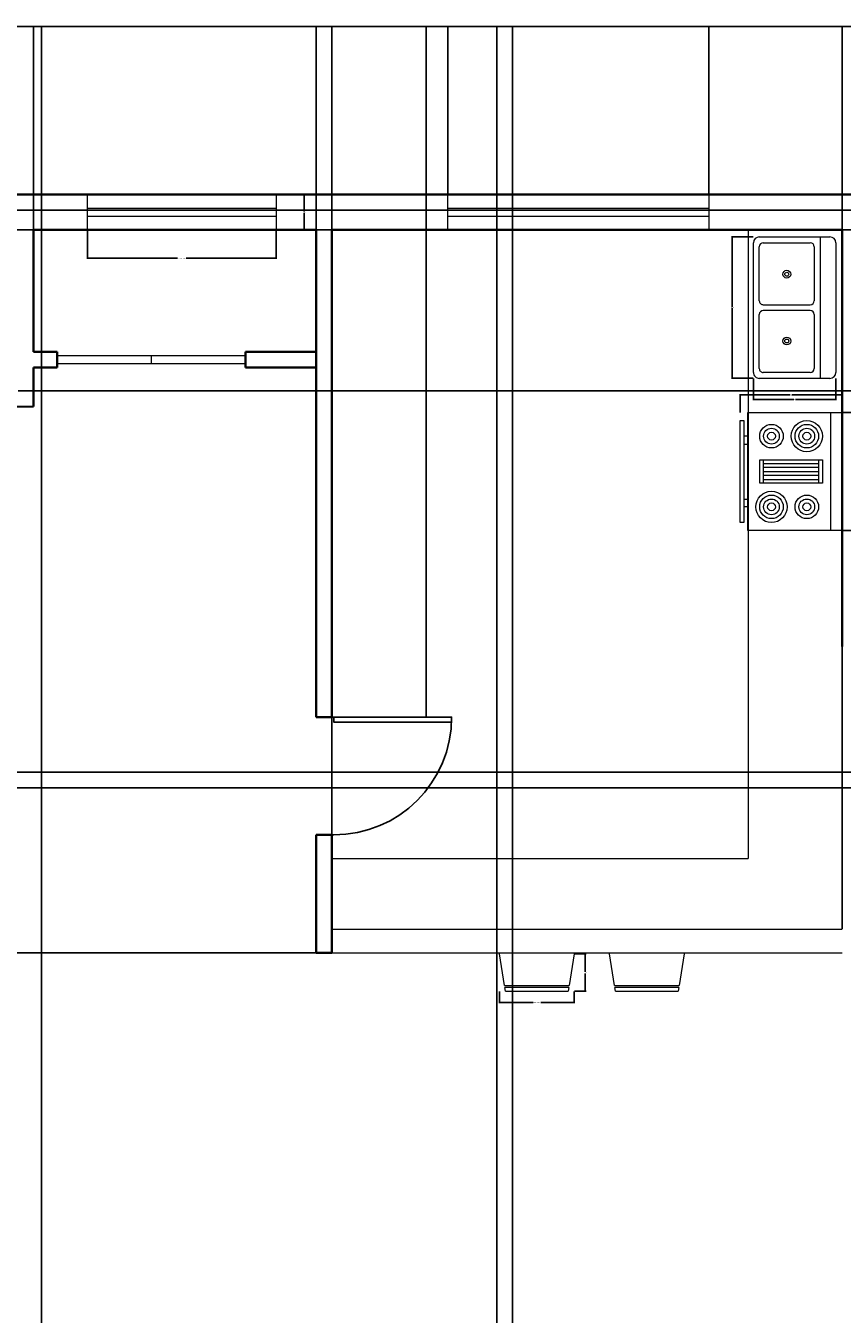
# Model space of a CAD drawing. Units: inches. Extents: x 2024 to 2965, y 1692 to 2308.
# Tile 7 of 8: x 2545 to 2753, y 1980 to 2308. Entities that reach past the tile are written whole.
import ezdxf

# ---------------------------------------------------------------- set-up
doc = ezdxf.new("R2010")
doc.units = ezdxf.units.IN
for name, color, linetype, lineweight in [('A-ANNO-DIMS', 2, 'Continuous', 18), ('A-DOOR', 3, 'Continuous', 25), ('A-EQPM', 6, 'Continuous', 18), ('A-FLOR-CASE', 33, 'Continuous', 20), ('A-FLOR-FIXT', 9, 'Continuous', 18), ('A-FURN', 8, 'Continuous', 18), ('A-GLAZ', 4, 'Continuous', 18), ('A-WALL', 7, 'Continuous', 35)]:
    doc.layers.add(name, color=color, linetype=linetype, lineweight=lineweight)
doc.styles.get("Standard").update_dxf_attribs({"font": 'arial.ttf'})
doc.dimstyles.get("Standard").update_dxf_attribs({"dimtxt": 0.18, "dimasz": 0.18, "dimexe": 0.18, "dimexo": 0.0625, "dimgap": 0.09, "dimtad": 0, "dimtih": 1, "dimtoh": 1, "dimdec": 4, "dimzin": 0, "dimdsep": 46, "dimtxsty": 'Standard', "dimcen": 0.09, "dimadec": 0, "dimazin": 0, "dimtfac": 1, "dimtdec": 4, "dimtofl": 0, "dimtmove": 0, "dimatfit": 3, "dimfxl": 1, "dimtolj": 1, "dimtzin": 0, "dimarcsym": 0})

# ---------------------------------------------------------------- blocks, each defined once
blk = doc.blocks.new('*U7')
for p, q in [((0, 0), (0, -6)), ((40, 0), (40, -6))]:
    blk.add_line(p, q)
blk.add_lwpolyline([(0, 0), (0, 40), (1.75, 40), (1.75, 0)], close=True)
blk.add_arc((0, 0), 40, 0, 90)
blk = doc.blocks.new('Range-Oven - 30 in top')
for p, q in [((0, -3), (30, -3)), ((12, -6), (18, -6)), ((13, -20), (13, -6)), ((14, -6), (14, -20)), ((15, -20), (15, -6)), ((16, -6), (16, -20)), ((17, -20), (17, -6)), ((18, -20), (12, -20)), ((6, -24), (6, -25)), ((8, -25), (8, -24)), ((22, -25), (22, -24)), ((24, -24), (24, -25))]:
    blk.add_line(p, q)
for points in [[(0, -24), (0, 0), (30, 0), (30, -24)], [(12, -21), (12, -5), (18, -5), (18, -21)], [(2, -26), (2, -25), (28, -25), (28, -26)]]:
    blk.add_lwpolyline(points, close=True)
for centre, radius in [((6, -9), 4), ((6, -9), 3), ((24, -9), 3), ((6, -9), 2), ((6, -9), 1), ((24, -9), 2), ((24, -9), 1), ((6, -18), 3), ((6, -18), 2), ((24, -18), 4), ((24, -18), 3), ((24, -18), 2), ((6, -18), 1), ((24, -18), 1)]:
    blk.add_circle(centre, radius)
blk = doc.blocks.new('Sink-double - 36 in top')
for p, q in [((-18, -4), (18, -4)), ((-0.75, -18.5), (-0.75, -6.5)), ((0.75, -6.5), (0.75, -18.5))]:
    blk.add_line(p, q)
for points in [[(-16.5, 0), (16.5, 0)], [(-18, -19.5), (-18, -1.5)], [(18, -1.5), (18, -19.5)], [(-16.5, -18.5), (-16.5, -6.5)], [(-15.5, -5.5), (-1.75, -5.5)], [(1.75, -5.5), (15.5, -5.5)], [(16.5, -6.5), (16.5, -18.5)], [(-1.75, -19.5), (-15.5, -19.5)], [(15.5, -19.5), (1.75, -19.5)], [(16.5, -21), (-16.5, -21)]]:
    blk.add_lwpolyline(points)
for centre, radius in [((-8.5, -12.5), 1), ((-8.5, -12.5), 0.5), ((8.5, -12.5), 1), ((8.5, -12.5), 0.5)]:
    blk.add_circle(centre, radius)
for centre, radius, start, end in [((-16.5, -1.5), 1.5, 90, 180), ((16.5, -1.5), 1.5, 0, 90), ((-15.5, -6.5), 1, 90, 180), ((-1.75, -6.5), 1, 0, 90), ((1.75, -6.5), 1, 90, 180), ((15.5, -6.5), 1, 0, 90), ((-16.5, -19.5), 1.5, 180, 270), ((-15.5, -18.5), 1, 180, 270), ((-1.75, -18.5), 1, 270, 0), ((1.75, -18.5), 1, 180, 270), ((15.5, -18.5), 1, 270, 0), ((16.5, -19.5), 1.5, 270, 0)]:
    blk.add_arc(centre, radius, start, end)
blk = doc.blocks.new('WIN-48-D9')
for p, q in [((0, 5.5), (48, 5.5)), ((0, 3.5), (48, 3.5))]:
    blk.add_line(p, q)
for points in [[(0, 0), (0, 9)], [(48, 9), (48, 0)]]:
    blk.add_lwpolyline(points)
blk = doc.blocks.new('COUNTER-STOOL')
for p, q in [((1.25, 1.5), (0, 9.5)), ((18.97, 9.5), (17.72, 1.5)), ((1.25, 1.5), (17.72, 1.5)), ((1.48, 0), (1.33, 1)), ((17.64, 1), (1.33, 1)), ((17.64, 1), (17.48, 0)), ((1.48, 0), (17.48, 0))]:
    blk.add_line(p, q)
blk = doc.blocks.new('*D31')
at = {"layer": 'A-ANNO-DIMS', "color": 0, "lineweight": -2, "transparency": 16777216}
for p, q in [((2560.66, 2255.71), (2560.66, 2248.39)), ((2608.66, 2255.71), (2608.66, 2248.39)), ((2560.84, 2248.57), (2583.54, 2248.57)), ((2608.48, 2248.57), (2585.78, 2248.57))]:
    blk.add_line(p, q, dxfattribs=at)
at = {"layer": 'A-ANNO-DIMS', "color": 0, "transparency": 16777216}
for points in [[(2560.84, 2248.6), (2560.84, 2248.54), (2560.66, 2248.57)], [(2608.48, 2248.6), (2608.48, 2248.54), (2608.66, 2248.57)]]:
    blk.add_solid(points, dxfattribs=at)
at = {"layer": 'Defpoints', "color": 0, "transparency": 16777216}
for p in [(2560.66, 2255.77), (2608.66, 2255.77), (2608.66, 2248.57)]:
    blk.add_point(p, dxfattribs=at)
at = {"layer": 'A-ANNO-DIMS', "color": 0, "transparency": 16777216, "insert": (2584.66, 2248.57), "char_height": 0.18, "attachment_point": 5}
blk.add_mtext('\\A1;WINDOW 48 TYP.', dxfattribs=at)
blk = doc.blocks.new('*D32')
at = {"layer": 'A-ANNO-DIMS', "color": 0, "lineweight": -2, "transparency": 16777216}
for p, q in [((2608.72, 2264.77), (2616.04, 2264.77)), ((2615.86, 2264.59), (2615.86, 2260.46)), ((2615.86, 2255.95), (2615.86, 2260.09)), ((2608.72, 2255.77), (2616.04, 2255.77))]:
    blk.add_line(p, q, dxfattribs=at)
at = {"layer": 'A-ANNO-DIMS', "color": 0, "transparency": 16777216}
for points in [[(2615.83, 2264.59), (2615.89, 2264.59), (2615.86, 2264.77)], [(2615.83, 2255.95), (2615.89, 2255.95), (2615.86, 2255.77)]]:
    blk.add_solid(points, dxfattribs=at)
at = {"layer": 'Defpoints', "color": 0, "transparency": 16777216}
for p in [(2608.66, 2264.77), (2615.86, 2264.77), (2608.66, 2255.77)]:
    blk.add_point(p, dxfattribs=at)
at = {"layer": 'A-ANNO-DIMS', "color": 0, "transparency": 16777216, "insert": (2615.86, 2260.27), "char_height": 0.18, "attachment_point": 5}
blk.add_mtext('\\A1;9 TYP.', dxfattribs=at)
blk = doc.blocks.new('*D51')
at = {"layer": 'A-ANNO-DIMS', "color": 0, "lineweight": -2, "transparency": 16777216}
for p, q in [((2665.63, 2061.9), (2665.63, 2058.94)), ((2684.6, 2061.9), (2684.6, 2058.94)), ((2665.81, 2059.12), (2674.13, 2059.12)), ((2684.42, 2059.12), (2676.11, 2059.12))]:
    blk.add_line(p, q, dxfattribs=at)
at = {"layer": 'A-ANNO-DIMS', "color": 0, "transparency": 16777216}
for points in [[(2665.81, 2059.15), (2665.81, 2059.09), (2665.63, 2059.12)], [(2684.42, 2059.15), (2684.42, 2059.09), (2684.6, 2059.12)]]:
    blk.add_solid(points, dxfattribs=at)
at = {"layer": 'Defpoints', "color": 0, "transparency": 16777216}
for p in [(2665.63, 2061.97), (2684.6, 2061.97), (2684.6, 2059.12)]:
    blk.add_point(p, dxfattribs=at)
at = {"layer": 'A-ANNO-DIMS', "color": 0, "transparency": 16777216, "insert": (2675.12, 2059.12), "char_height": 0.18, "attachment_point": 5}
blk.add_mtext('\\A1;STOOL 19 TYP.', dxfattribs=at)
blk = doc.blocks.new('*D52')
at = {"layer": 'A-ANNO-DIMS', "color": 0, "lineweight": -2, "transparency": 16777216}
for p, q in [((2684.66, 2071.47), (2687.63, 2071.47)), ((2687.45, 2071.29), (2687.45, 2066.9)), ((2687.45, 2062.15), (2687.45, 2066.53)), ((2684.66, 2061.97), (2687.63, 2061.97))]:
    blk.add_line(p, q, dxfattribs=at)
at = {"layer": 'A-ANNO-DIMS', "color": 0, "transparency": 16777216}
for points in [[(2687.42, 2071.29), (2687.48, 2071.29), (2687.45, 2071.47)], [(2687.42, 2062.15), (2687.48, 2062.15), (2687.45, 2061.97)]]:
    blk.add_solid(points, dxfattribs=at)
at = {"layer": 'Defpoints', "color": 0, "transparency": 16777216}
for p in [(2684.6, 2071.47), (2687.45, 2071.47), (2684.6, 2061.97)]:
    blk.add_point(p, dxfattribs=at)
at = {"layer": 'A-ANNO-DIMS', "color": 0, "transparency": 16777216, "insert": (2687.45, 2066.72), "char_height": 0.18, "attachment_point": 5}
blk.add_mtext('\\A1;10 TYP.', dxfattribs=at)
blk = doc.blocks.new('*D71')
at = {"layer": 'A-ANNO-DIMS', "color": 0, "lineweight": -2, "transparency": 16777216}
for p, q in [((2752.94, 2209.27), (2757.56, 2209.27)), ((2757.38, 2209.09), (2757.38, 2194.46)), ((2757.38, 2179.45), (2757.38, 2194.09)), ((2752.94, 2179.27), (2757.56, 2179.27))]:
    blk.add_line(p, q, dxfattribs=at)
at = {"layer": 'A-ANNO-DIMS', "color": 0, "transparency": 16777216}
for points in [[(2757.35, 2209.09), (2757.41, 2209.09), (2757.38, 2209.27)], [(2757.35, 2179.45), (2757.41, 2179.45), (2757.38, 2179.27)]]:
    blk.add_solid(points, dxfattribs=at)
at = {"layer": 'Defpoints', "color": 0, "transparency": 16777216}
for p in [(2752.88, 2209.27), (2752.88, 2179.27), (2757.38, 2179.27)]:
    blk.add_point(p, dxfattribs=at)
at = {"layer": 'A-ANNO-DIMS', "color": 0, "transparency": 16777216, "insert": (2757.38, 2194.27), "char_height": 0.18, "attachment_point": 5}
blk.add_mtext('\\A1;RANGE 30', dxfattribs=at)
blk = doc.blocks.new('*D72')
at = {"layer": 'A-ANNO-DIMS', "color": 0, "lineweight": -2, "transparency": 16777216}
for p, q in [((2726.88, 2209.33), (2726.88, 2213.95)), ((2727.06, 2213.77), (2739.66, 2213.77)), ((2752.7, 2213.77), (2740.1, 2213.77)), ((2752.88, 2209.33), (2752.88, 2213.95))]:
    blk.add_line(p, q, dxfattribs=at)
at = {"layer": 'A-ANNO-DIMS', "color": 0, "transparency": 16777216}
for points in [[(2727.06, 2213.8), (2727.06, 2213.74), (2726.88, 2213.77)], [(2752.7, 2213.8), (2752.7, 2213.74), (2752.88, 2213.77)]]:
    blk.add_solid(points, dxfattribs=at)
at = {"layer": 'Defpoints', "color": 0, "transparency": 16777216}
for p in [(2752.88, 2213.77), (2726.88, 2209.27), (2752.88, 2209.27)]:
    blk.add_point(p, dxfattribs=at)
at = {"layer": 'A-ANNO-DIMS', "color": 0, "transparency": 16777216, "insert": (2739.88, 2213.77), "char_height": 0.18, "attachment_point": 5}
blk.add_mtext('\\A1;26', dxfattribs=at)
blk = doc.blocks.new('*D73')
at = {"layer": 'A-ANNO-DIMS', "color": 0, "lineweight": -2, "transparency": 16777216}
for p, q in [((2730.21, 2253.99), (2724.69, 2253.99)), ((2724.87, 2253.81), (2724.87, 2236.17)), ((2724.87, 2218.17), (2724.87, 2235.81)), ((2730.21, 2217.99), (2724.69, 2217.99))]:
    blk.add_line(p, q, dxfattribs=at)
at = {"layer": 'A-ANNO-DIMS', "color": 0, "transparency": 16777216}
for points in [[(2724.84, 2253.81), (2724.9, 2253.81), (2724.87, 2253.99)], [(2724.84, 2218.17), (2724.9, 2218.17), (2724.87, 2217.99)]]:
    blk.add_solid(points, dxfattribs=at)
at = {"layer": 'Defpoints', "color": 0, "transparency": 16777216}
for p in [(2730.27, 2253.99), (2724.87, 2217.99), (2730.27, 2217.99)]:
    blk.add_point(p, dxfattribs=at)
at = {"layer": 'A-ANNO-DIMS', "color": 0, "transparency": 16777216, "insert": (2724.87, 2235.99), "char_height": 0.18, "attachment_point": 5}
blk.add_mtext('\\A1;SINK 36', dxfattribs=at)
blk = doc.blocks.new('*D74')
at = {"layer": 'A-ANNO-DIMS', "color": 0, "lineweight": -2, "transparency": 16777216}
for p, q in [((2730.27, 2217.93), (2730.27, 2212.41)), ((2751.27, 2217.93), (2751.27, 2212.41)), ((2730.45, 2212.59), (2740.57, 2212.59)), ((2751.09, 2212.59), (2740.98, 2212.59))]:
    blk.add_line(p, q, dxfattribs=at)
at = {"layer": 'A-ANNO-DIMS', "color": 0, "transparency": 16777216}
for points in [[(2730.45, 2212.62), (2730.45, 2212.56), (2730.27, 2212.59)], [(2751.09, 2212.62), (2751.09, 2212.56), (2751.27, 2212.59)]]:
    blk.add_solid(points, dxfattribs=at)
at = {"layer": 'Defpoints', "color": 0, "transparency": 16777216}
for p in [(2730.27, 2217.99), (2751.27, 2217.99), (2751.27, 2212.59)]:
    blk.add_point(p, dxfattribs=at)
at = {"layer": 'A-ANNO-DIMS', "color": 0, "transparency": 16777216, "insert": (2740.77, 2212.59), "char_height": 0.18, "attachment_point": 5}
blk.add_mtext('\\A1;21', dxfattribs=at)
blk = doc.blocks.new('*D76')
at = {"layer": 'A-ANNO-DIMS', "color": 0, "lineweight": -2, "transparency": 16777216}
for p, q in [((2718.97, 2264.77), (2964.97, 2264.77)), ((2964.79, 2264.59), (2964.79, 2000.12)), ((2964.79, 1735.28), (2964.79, 1999.75)), ((2515.28, 1735.1), (2964.97, 1735.1))]:
    blk.add_line(p, q, dxfattribs=at)
at = {"layer": 'A-ANNO-DIMS', "color": 0, "transparency": 16777216}
for points in [[(2964.76, 2264.59), (2964.82, 2264.59), (2964.79, 2264.77)], [(2964.76, 1735.28), (2964.82, 1735.28), (2964.79, 1735.1)]]:
    blk.add_solid(points, dxfattribs=at)
at = {"layer": 'Defpoints', "color": 0, "transparency": 16777216}
for p in [(2718.91, 2264.77), (2515.22, 1735.1), (2964.79, 1735.1)]:
    blk.add_point(p, dxfattribs=at)
at = {"layer": 'A-ANNO-DIMS', "color": 0, "transparency": 16777216, "insert": (2964.79, 1999.94), "char_height": 0.18, "attachment_point": 5}
blk.add_mtext('\\A1;529.7', dxfattribs=at)
blk = doc.blocks.new('*D82')
at = {"layer": 'A-ANNO-DIMS', "color": 0, "lineweight": -2, "transparency": 16777216}
for p, q in [((2546.91, 2255.84), (2546.91, 2307.73)), ((2547.09, 2307.55), (2582.69, 2307.55)), ((2618.73, 2307.55), (2583.12, 2307.55)), ((2618.91, 2255.84), (2618.91, 2307.73))]:
    blk.add_line(p, q, dxfattribs=at)
at = {"layer": 'A-ANNO-DIMS', "color": 0, "transparency": 16777216}
for points in [[(2547.09, 2307.58), (2547.09, 2307.52), (2546.91, 2307.55)], [(2618.73, 2307.58), (2618.73, 2307.52), (2618.91, 2307.55)]]:
    blk.add_solid(points, dxfattribs=at)
at = {"layer": 'Defpoints', "color": 0, "transparency": 16777216}
for p in [(2618.91, 2307.55), (2546.91, 2255.77), (2618.91, 2255.77)]:
    blk.add_point(p, dxfattribs=at)
at = {"layer": 'A-ANNO-DIMS', "color": 0, "transparency": 16777216, "insert": (2582.91, 2307.55), "char_height": 0.18, "attachment_point": 5}
blk.add_mtext('\\A1;72', dxfattribs=at)
blk = doc.blocks.new('*D83')
at = {"layer": 'A-ANNO-DIMS', "color": 0, "lineweight": -2, "transparency": 16777216}
for p, q in [((2622.91, 2077.84), (2622.91, 2307.73)), ((2623.09, 2307.55), (2687.63, 2307.55)), ((2752.73, 2307.55), (2688.19, 2307.55)), ((2752.91, 2077.84), (2752.91, 2307.73))]:
    blk.add_line(p, q, dxfattribs=at)
at = {"layer": 'A-ANNO-DIMS', "color": 0, "transparency": 16777216}
for points in [[(2623.09, 2307.58), (2623.09, 2307.52), (2622.91, 2307.55)], [(2752.73, 2307.58), (2752.73, 2307.52), (2752.91, 2307.55)]]:
    blk.add_solid(points, dxfattribs=at)
at = {"layer": 'Defpoints', "color": 0, "transparency": 16777216}
for p in [(2752.91, 2307.55), (2622.91, 2077.77), (2752.91, 2077.77)]:
    blk.add_point(p, dxfattribs=at)
at = {"layer": 'A-ANNO-DIMS', "color": 0, "transparency": 16777216, "insert": (2687.91, 2307.55), "char_height": 0.18, "attachment_point": 5}
blk.add_mtext('\\A1;130', dxfattribs=at)
blk = doc.blocks.new('*D84')
at = {"layer": 'A-ANNO-DIMS', "color": 0, "lineweight": -2, "transparency": 16777216}
for p, q in [((2618.84, 2255.77), (2024.5, 2255.77)), ((2024.68, 2255.59), (2024.68, 2163.96)), ((2024.68, 2071.95), (2024.68, 2163.59)), ((2618.84, 2071.77), (2024.5, 2071.77))]:
    blk.add_line(p, q, dxfattribs=at)
at = {"layer": 'A-ANNO-DIMS', "color": 0, "transparency": 16777216}
for points in [[(2024.65, 2255.59), (2024.71, 2255.59), (2024.68, 2255.77)], [(2024.65, 2071.95), (2024.71, 2071.95), (2024.68, 2071.77)]]:
    blk.add_solid(points, dxfattribs=at)
at = {"layer": 'Defpoints', "color": 0, "transparency": 16777216}
for p in [(2024.68, 2255.77), (2618.91, 2255.77), (2618.91, 2071.77)]:
    blk.add_point(p, dxfattribs=at)
at = {"layer": 'A-ANNO-DIMS', "color": 0, "transparency": 16777216, "insert": (2024.68, 2163.77), "char_height": 0.18, "attachment_point": 5}
blk.add_mtext('\\A1;184', dxfattribs=at)
blk = doc.blocks.new('*D85')
at = {"layer": 'A-ANNO-DIMS', "color": 0, "lineweight": -2, "transparency": 16777216}
for p, q in [((2622.91, 2131.84), (2622.91, 2307.73)), ((2623.09, 2307.55), (2634.69, 2307.55)), ((2646.73, 2307.55), (2635.13, 2307.55)), ((2646.91, 2131.84), (2646.91, 2307.73))]:
    blk.add_line(p, q, dxfattribs=at)
at = {"layer": 'A-ANNO-DIMS', "color": 0, "transparency": 16777216}
for points in [[(2623.09, 2307.58), (2623.09, 2307.52), (2622.91, 2307.55)], [(2646.73, 2307.58), (2646.73, 2307.52), (2646.91, 2307.55)]]:
    blk.add_solid(points, dxfattribs=at)
at = {"layer": 'Defpoints', "color": 0, "transparency": 16777216}
for p in [(2646.91, 2307.55), (2622.91, 2131.77), (2646.91, 2131.77)]:
    blk.add_point(p, dxfattribs=at)
at = {"layer": 'A-ANNO-DIMS', "color": 0, "transparency": 16777216, "insert": (2634.91, 2307.55), "char_height": 0.18, "attachment_point": 5}
blk.add_mtext('\\A1;24', dxfattribs=at)
blk = doc.blocks.new('*D86')
at = {"layer": 'A-ANNO-DIMS', "color": 0, "lineweight": -2, "transparency": 16777216}
for p, q in [((2652.45, 2264.84), (2652.45, 2307.73)), ((2652.63, 2307.55), (2685.28, 2307.55)), ((2718.73, 2307.55), (2686.07, 2307.55)), ((2718.91, 2264.84), (2718.91, 2307.73))]:
    blk.add_line(p, q, dxfattribs=at)
at = {"layer": 'A-ANNO-DIMS', "color": 0, "transparency": 16777216}
for points in [[(2652.63, 2307.58), (2652.63, 2307.52), (2652.45, 2307.55)], [(2718.73, 2307.58), (2718.73, 2307.52), (2718.91, 2307.55)]]:
    blk.add_solid(points, dxfattribs=at)
at = {"layer": 'Defpoints', "color": 0, "transparency": 16777216}
for p in [(2718.91, 2307.55), (2652.45, 2264.77), (2718.91, 2264.77)]:
    blk.add_point(p, dxfattribs=at)
at = {"layer": 'A-ANNO-DIMS', "color": 0, "transparency": 16777216, "insert": (2685.68, 2307.55), "char_height": 0.18, "attachment_point": 5}
blk.add_mtext('\\A1;66.45', dxfattribs=at)
blk = doc.blocks.new('*D88')
at = {"layer": 'A-ANNO-DIMS', "color": 0, "lineweight": -2, "transparency": 16777216}
for p, q in [((2817.84, 2260.77), (2024.5, 2260.77)), ((2024.68, 2260.59), (2024.68, 2189.46)), ((2024.68, 2117.95), (2024.68, 2189.09)), ((2817.84, 2117.77), (2024.5, 2117.77))]:
    blk.add_line(p, q, dxfattribs=at)
at = {"layer": 'A-ANNO-DIMS', "color": 0, "transparency": 16777216}
for points in [[(2024.65, 2260.59), (2024.71, 2260.59), (2024.68, 2260.77)], [(2024.65, 2117.95), (2024.71, 2117.95), (2024.68, 2117.77)]]:
    blk.add_solid(points, dxfattribs=at)
at = {"layer": 'Defpoints', "color": 0, "transparency": 16777216}
for p in [(2817.91, 2260.77), (2024.68, 2117.77), (2817.91, 2117.77)]:
    blk.add_point(p, dxfattribs=at)
at = {"layer": 'A-ANNO-DIMS', "color": 0, "transparency": 16777216, "insert": (2024.68, 2189.27), "char_height": 0.18, "attachment_point": 5}
blk.add_mtext('\\A1;143', dxfattribs=at)
blk = doc.blocks.new('*D98')
at = {"layer": 'A-ANNO-DIMS', "color": 0, "lineweight": -2, "transparency": 16777216}
for p, q in [((2422.91, 1973.84), (2422.91, 2307.73)), ((2423.09, 2307.55), (2543.62, 2307.55)), ((2664.73, 2307.55), (2544.2, 2307.55)), ((2664.91, 1956.85), (2664.91, 2307.73))]:
    blk.add_line(p, q, dxfattribs=at)
at = {"layer": 'A-ANNO-DIMS', "color": 0, "transparency": 16777216}
for points in [[(2423.09, 2307.58), (2423.09, 2307.52), (2422.91, 2307.55)], [(2664.73, 2307.58), (2664.73, 2307.52), (2664.91, 2307.55)]]:
    blk.add_solid(points, dxfattribs=at)
at = {"layer": 'Defpoints', "color": 0, "transparency": 16777216}
for p in [(2664.91, 2307.55), (2422.91, 1973.77), (2664.91, 1956.79)]:
    blk.add_point(p, dxfattribs=at)
at = {"layer": 'A-ANNO-DIMS', "color": 0, "transparency": 16777216, "insert": (2543.91, 2307.55), "char_height": 0.18, "attachment_point": 5}
blk.add_mtext('\\A1;242', dxfattribs=at)
blk = doc.blocks.new('*D99')
at = {"layer": 'A-ANNO-DIMS', "color": 0, "lineweight": -2, "transparency": 16777216}
for p, q in [((2668.91, 1952.85), (2668.91, 2307.73)), ((2669.09, 2307.55), (2749.48, 2307.55)), ((2830.78, 2307.55), (2750.39, 2307.55)), ((2830.96, 1952.97), (2830.96, 2307.73))]:
    blk.add_line(p, q, dxfattribs=at)
at = {"layer": 'A-ANNO-DIMS', "color": 0, "transparency": 16777216}
for points in [[(2669.09, 2307.58), (2669.09, 2307.52), (2668.91, 2307.55)], [(2830.78, 2307.58), (2830.78, 2307.52), (2830.96, 2307.55)]]:
    blk.add_solid(points, dxfattribs=at)
at = {"layer": 'Defpoints', "color": 0, "transparency": 16777216}
for p in [(2830.96, 2307.55), (2668.91, 1952.79), (2830.96, 1952.91)]:
    blk.add_point(p, dxfattribs=at)
at = {"layer": 'A-ANNO-DIMS', "color": 0, "transparency": 16777216, "insert": (2749.93, 2307.55), "char_height": 0.18, "attachment_point": 5}
blk.add_mtext('\\A1;162.06', dxfattribs=at)
blk = doc.blocks.new('*D101')
at = {"layer": 'A-ANNO-DIMS', "color": 0, "lineweight": -2, "transparency": 16777216}
for p, q in [((2917.96, 2113.77), (2024.5, 2113.77)), ((2024.68, 2113.59), (2024.68, 2035.52)), ((2024.68, 1957.09), (2024.68, 2035.16)), ((2917.96, 1956.91), (2024.5, 1956.91))]:
    blk.add_line(p, q, dxfattribs=at)
at = {"layer": 'A-ANNO-DIMS', "color": 0, "transparency": 16777216}
for points in [[(2024.65, 2113.59), (2024.71, 2113.59), (2024.68, 2113.77)], [(2024.65, 1957.09), (2024.71, 1957.09), (2024.68, 1956.91)]]:
    blk.add_solid(points, dxfattribs=at)
at = {"layer": 'Defpoints', "color": 0, "transparency": 16777216}
for p in [(2024.68, 2113.77), (2918.02, 2113.77), (2918.02, 1956.91)]:
    blk.add_point(p, dxfattribs=at)
at = {"layer": 'A-ANNO-DIMS', "color": 0, "transparency": 16777216, "insert": (2024.68, 2035.34), "char_height": 0.18, "attachment_point": 5}
blk.add_mtext('\\A1;156.87', dxfattribs=at)
blk = doc.blocks.new('*D108')
at = {"layer": 'A-ANNO-DIMS', "color": 0, "lineweight": -2, "transparency": 16777216}
for p, q in [((2542.97, 2255.77), (2964.97, 2255.77)), ((2964.79, 2255.59), (2964.79, 2235.45)), ((2964.79, 2214.95), (2964.79, 2235.09)), ((2542.97, 2214.77), (2964.97, 2214.77))]:
    blk.add_line(p, q, dxfattribs=at)
at = {"layer": 'A-ANNO-DIMS', "color": 0, "transparency": 16777216}
for points in [[(2964.76, 2255.59), (2964.82, 2255.59), (2964.79, 2255.77)], [(2964.76, 2214.95), (2964.82, 2214.95), (2964.79, 2214.77)]]:
    blk.add_solid(points, dxfattribs=at)
at = {"layer": 'Defpoints', "color": 0, "transparency": 16777216}
for p in [(2542.91, 2255.77), (2542.91, 2214.77), (2964.79, 2214.77)]:
    blk.add_point(p, dxfattribs=at)
at = {"layer": 'A-ANNO-DIMS', "color": 0, "transparency": 16777216, "insert": (2964.79, 2235.27), "char_height": 0.18, "attachment_point": 5}
blk.add_mtext('\\A1;41', dxfattribs=at)
blk = doc.blocks.new('*D114')
at = {"layer": 'A-ANNO-DIMS', "color": 0, "lineweight": -2, "transparency": 16777216}
for p, q in [((2428.91, 1761.01), (2428.91, 2307.73)), ((2429.09, 2307.55), (2488.63, 2307.55)), ((2548.73, 2307.55), (2489.19, 2307.55)), ((2548.91, 1761.01), (2548.91, 2307.73))]:
    blk.add_line(p, q, dxfattribs=at)
at = {"layer": 'A-ANNO-DIMS', "color": 0, "transparency": 16777216}
for points in [[(2429.09, 2307.58), (2429.09, 2307.52), (2428.91, 2307.55)], [(2548.73, 2307.58), (2548.73, 2307.52), (2548.91, 2307.55)]]:
    blk.add_solid(points, dxfattribs=at)
at = {"layer": 'Defpoints', "color": 0, "transparency": 16777216}
for p in [(2548.91, 2307.55), (2428.91, 1760.95), (2548.91, 1760.95)]:
    blk.add_point(p, dxfattribs=at)
at = {"layer": 'A-ANNO-DIMS', "color": 0, "transparency": 16777216, "insert": (2488.91, 2307.55), "char_height": 0.18, "attachment_point": 5}
blk.add_mtext('\\A1;120', dxfattribs=at)
blk = doc.blocks.new('*D117')
at = {"layer": 'A-ANNO-DIMS', "color": 0, "lineweight": -2, "transparency": 16777216}
for p, q in [((2622.91, 2255.84), (2622.91, 2307.73)), ((2623.09, 2307.55), (2637.21, 2307.55)), ((2652.27, 2307.55), (2638.14, 2307.55)), ((2652.45, 2264.84), (2652.45, 2307.73))]:
    blk.add_line(p, q, dxfattribs=at)
at = {"layer": 'A-ANNO-DIMS', "color": 0, "transparency": 16777216}
for points in [[(2623.09, 2307.58), (2623.09, 2307.52), (2622.91, 2307.55)], [(2652.27, 2307.58), (2652.27, 2307.52), (2652.45, 2307.55)]]:
    blk.add_solid(points, dxfattribs=at)
at = {"layer": 'Defpoints', "color": 0, "transparency": 16777216}
for p in [(2622.91, 2307.55), (2652.45, 2264.77), (2622.91, 2255.77)]:
    blk.add_point(p, dxfattribs=at)
at = {"layer": 'A-ANNO-DIMS', "color": 0, "transparency": 16777216, "insert": (2637.68, 2307.55), "char_height": 0.18, "attachment_point": 5}
blk.add_mtext('\\A1;29.546', dxfattribs=at)

msp = doc.modelspace()

# ---------------------------------------------------------------- linework, layer by layer
at = {"layer": 'A-FLOR-CASE'}
for p, q in [((2646.9061, 2131.7736), (2646.9061, 2255.7736)), ((2728.9061, 2255.7736), (2728.9061, 2149.7736)), ((2728.9061, 2149.7736), (2728.9061, 2119.7736)), ((2622.9061, 2131.7736), (2646.9061, 2131.7736)), ((2728.9061, 2119.7736), (2728.9061, 2095.7736)), ((2622.9061, 2095.7736), (2728.9061, 2095.7736)), ((2622.9061, 2077.7736), (2752.9061, 2077.7736)), ((2622.9061, 2071.7736), (2752.9061, 2071.7736))]:
    msp.add_line(p, q, dxfattribs=at)
at = {"layer": 'A-GLAZ'}
for p, q in [((2652.4523, 2261.2736), (2718.9061, 2261.2736)), ((2652.4523, 2259.2736), (2718.9061, 2259.2736)), ((2552.9061, 2223.7827), (2600.9061, 2223.7827)), ((2576.9061, 2221.7827), (2576.9061, 2223.7827)), ((2552.9061, 2221.7827), (2600.9061, 2221.7827))]:
    msp.add_line(p, q, dxfattribs=at)
for points in [[(2652.4523, 2255.7736), (2652.4523, 2264.7736)], [(2718.9061, 2264.7736), (2718.9061, 2255.7736)], [(2552.9061, 2220.7696), (2552.9061, 2224.7696)], [(2600.9061, 2224.7696), (2600.9061, 2220.7696)]]:
    msp.add_lwpolyline(points, dxfattribs=at)
at = {"layer": 'A-WALL'}
for p, q in [((2161.9061, 2264.7736), (2821.9061, 2264.7736)), ((2546.9061, 2255.7736), (2618.9061, 2255.7736)), ((2546.9061, 2224.7696), (2546.9061, 2255.7736)), ((2618.9061, 2131.7736), (2618.9061, 2255.7736)), ((2622.9061, 2131.7736), (2622.9061, 2255.7736)), ((2622.9061, 2255.7736), (2752.9061, 2255.7736)), ((2752.9061, 2255.7736), (2752.9061, 2149.7736)), ((2546.9061, 2224.7696), (2552.9061, 2224.7696)), ((2552.9061, 2224.7696), (2552.9061, 2220.7696)), ((2600.9061, 2224.7696), (2600.9061, 2220.7696)), ((2600.9061, 2224.7696), (2618.9061, 2224.7696)), ((2546.9061, 2210.7871), (2546.9061, 2220.7696)), ((2546.9061, 2220.7696), (2552.9061, 2220.7696)), ((2600.9061, 2220.7696), (2618.9061, 2220.7696)), ((2512.9058, 2210.6382), (2546.9061, 2210.7871)), ((2618.9061, 2131.7736), (2622.9061, 2131.7736)), ((2618.9061, 2101.7736), (2622.9061, 2101.7736)), ((2618.9061, 2071.7736), (2618.9061, 2101.7736)), ((2622.9061, 2101.7736), (2622.9061, 2071.7736)), ((2622.9061, 2071.7736), (2618.9061, 2071.7736))]:
    msp.add_line(p, q, dxfattribs=at)

# ---------------------------------------------------------------- block references
at = {"layer": 'A-DOOR', "xscale": 0.75, "yscale": 0.75, "zscale": 0.75, "rotation": 270}
msp.add_blockref('*U7', (2623.4061, 2131.7736), dxfattribs=at)
at = {"layer": 'A-EQPM', "rotation": 270}
msp.add_blockref('Range-Oven - 30 in top', (2752.8769, 2209.2724), dxfattribs=at)
at = {"layer": 'A-FLOR-FIXT', "rotation": 270}
msp.add_blockref('Sink-double - 36 in top', (2751.2749, 2235.9895), dxfattribs=at)
at = {"layer": 'A-FURN'}
for p in [(2665.632, 2061.966), (2693.632, 2061.966)]:
    msp.add_blockref('COUNTER-STOOL', p, dxfattribs=at)
at = {"layer": 'A-GLAZ'}
msp.add_blockref('WIN-48-D9', (2560.661, 2255.774), dxfattribs=at)

# ---------------------------------------------------------------- dimensions: what is measured, and where the dimension line sits
at = {"layer": 'A-ANNO-DIMS'}
for base, p1, p2, override, picture, middle in [((2664.9061, 2307.5486), (2422.9061, 1973.7736), (2664.9061, 1956.7881), {"dimdec": 0, "dimlfac": 1, "dimrnd": 0, "dimzin": 0, "dimdsep": 46, "dimlunit": 2}, '*D98', (2543.9061, 2307.5486)), ((2548.9061, 2307.5486), (2428.9061, 1760.9504), (2548.9061, 1760.9504), {"dimdec": 0, "dimlfac": 1, "dimrnd": 0, "dimzin": 0, "dimdsep": 46, "dimlunit": 2}, '*D114', (2488.9061, 2307.5486)), ((2618.9061, 2307.5486), (2546.9061, 2255.7736), (2618.9061, 2255.7736), {"dimdec": 0, "dimlfac": 1, "dimrnd": 0, "dimzin": 0, "dimdsep": 46, "dimlunit": 2}, '*D82', (2582.9061, 2307.5486)), ((2752.9061, 2307.5486), (2622.9061, 2077.7736), (2752.9061, 2077.7736), {"dimdec": 0, "dimlfac": 1, "dimrnd": 0, "dimzin": 0, "dimdsep": 46, "dimlunit": 2}, '*D83', (2687.9061, 2307.5486)), ((2646.9061, 2307.5486), (2622.9061, 2131.7736), (2646.9061, 2131.7736), {"dimdec": 0, "dimlfac": 1, "dimrnd": 0, "dimzin": 0, "dimdsep": 46, "dimlunit": 2}, '*D85', (2634.9061, 2307.5486)), ((2622.9061, 2307.5486), (2652.4523, 2264.7736), (2622.9061, 2255.7736), {"dimdec": 3, "dimlfac": 1, "dimrnd": 0, "dimzin": 0, "dimdsep": 46, "dimlunit": 2}, '*D117', (2637.6792, 2307.5486)), ((2718.9061, 2307.5486), (2652.4523, 2264.7736), (2718.9061, 2264.7736), {"dimdec": 2, "dimlfac": 1, "dimrnd": 0, "dimzin": 0, "dimdsep": 46, "dimlunit": 2}, '*D86', (2685.6792, 2307.5486)), ((2830.9627, 2307.5486), (2668.9061, 1952.7881), (2830.9627, 1952.9082), {"dimdec": 2, "dimlfac": 1, "dimrnd": 0, "dimzin": 0, "dimdsep": 46, "dimlunit": 2}, '*D99', (2749.9344, 2307.5486)), ((2751.2749, 2212.5895), (2730.2749, 2217.9895), (2751.2749, 2217.9895), {"dimdec": 0, "dimlfac": 1, "dimrnd": 0, "dimzin": 0, "dimdsep": 46, "dimlunit": 2}, '*D74', (2740.7749, 2212.5895)), ((2752.8769, 2213.7724), (2726.8769, 2209.2724), (2752.8769, 2209.2724), {"dimdec": 0, "dimlfac": 1, "dimrnd": 0, "dimzin": 0, "dimdsep": 46, "dimlunit": 2}, '*D72', (2739.8769, 2213.7724))]:
    dim = msp.add_linear_dim(base=base, p1=p1, p2=p2, dimstyle='Standard', override=override, dxfattribs=at)
    dim.commit()
    dim.dimension.update_dxf_attribs({"geometry": picture, "text_midpoint": middle})
for base, p1, p2, override, picture, middle in [((2964.7942, 1735.0986), (2718.9061, 2264.7736), (2515.2195, 1735.0986), {"dimdec": 1, "dimlfac": 1, "dimrnd": 0, "dimzin": 0, "dimdsep": 46, "dimlunit": 2}, '*D76', (2964.7942, 1999.9361)), ((2024.6844, 2117.7736), (2817.9061, 2260.7736), (2817.9061, 2117.7736), {"dimdec": 0, "dimlfac": 1, "dimrnd": 0, "dimzin": 0, "dimdsep": 46, "dimlunit": 2}, '*D88', (2024.6844, 2189.2736)), ((2024.6844, 2255.7736), (2618.9061, 2071.7736), (2618.9061, 2255.7736), {"dimdec": 0, "dimlfac": 1, "dimrnd": 0, "dimzin": 0, "dimdsep": 46, "dimlunit": 2}, '*D84', (2024.6844, 2163.7736)), ((2964.7942, 2214.7696), (2542.9061, 2255.7736), (2542.9061, 2214.7696), {"dimdec": 0, "dimlfac": 1, "dimrnd": 0, "dimzin": 0, "dimdsep": 46, "dimlunit": 2}, '*D108', (2964.7942, 2235.2716)), ((2024.6844, 2113.7736), (2918.0192, 1956.9082), (2918.0192, 2113.7736), {"dimdec": 2, "dimlfac": 1, "dimrnd": 0, "dimzin": 0, "dimdsep": 46, "dimlunit": 2}, '*D101', (2024.6844, 2035.3409))]:
    dim = msp.add_linear_dim(base=base, p1=p1, p2=p2, angle=90, dimstyle='Standard', override=override, dxfattribs=at)
    dim.commit()
    dim.dimension.update_dxf_attribs({"geometry": picture, "text_midpoint": middle})
for base, p1, p2, angle, text, picture, middle in [((2615.8609, 2264.7736), (2608.6609, 2255.7736), (2608.6609, 2264.7736), 90, '<> TYP.', '*D32', (2615.8609, 2260.2736)), ((2724.8749, 2217.9895), (2730.2749, 2253.9895), (2730.2749, 2217.9895), 270, 'SINK <>', '*D73', (2724.8749, 2235.9895)), ((2757.3769, 2179.2724), (2752.8769, 2209.2724), (2752.8769, 2179.2724), 270, 'RANGE <>', '*D71', (2757.3769, 2194.2724)), ((2687.447, 2071.468), (2684.6016, 2061.9656), (2684.6016, 2071.468), 90, '<> TYP.', '*D52', (2687.447, 2066.7168))]:
    dim = msp.add_linear_dim(base=base, p1=p1, p2=p2, angle=angle, text=text, dimstyle='Standard', override={"dimdec": 0, "dimlfac": 1, "dimrnd": 0, "dimzin": 0, "dimdsep": 46, "dimlunit": 2}, dxfattribs=at)
    dim.commit()
    dim.dimension.update_dxf_attribs({"geometry": picture, "text_midpoint": middle})
for base, p1, p2, text, picture, middle in [((2608.6609, 2248.5736), (2560.6609, 2255.7736), (2608.6609, 2255.7736), 'WINDOW <> TYP.', '*D31', (2584.6609, 2248.5736)), ((2684.6016, 2059.1202), (2665.6321, 2061.9656), (2684.6016, 2061.9656), 'STOOL <> TYP.', '*D51', (2675.1169, 2059.1202))]:
    dim = msp.add_linear_dim(base=base, p1=p1, p2=p2, text=text, dimstyle='Standard', override={"dimdec": 0, "dimlfac": 1, "dimrnd": 0, "dimzin": 0, "dimdsep": 46, "dimlunit": 2}, dxfattribs=at)
    dim.commit()
    dim.dimension.update_dxf_attribs({"geometry": picture, "text_midpoint": middle})

doc.saveas('drawing.dxf')
